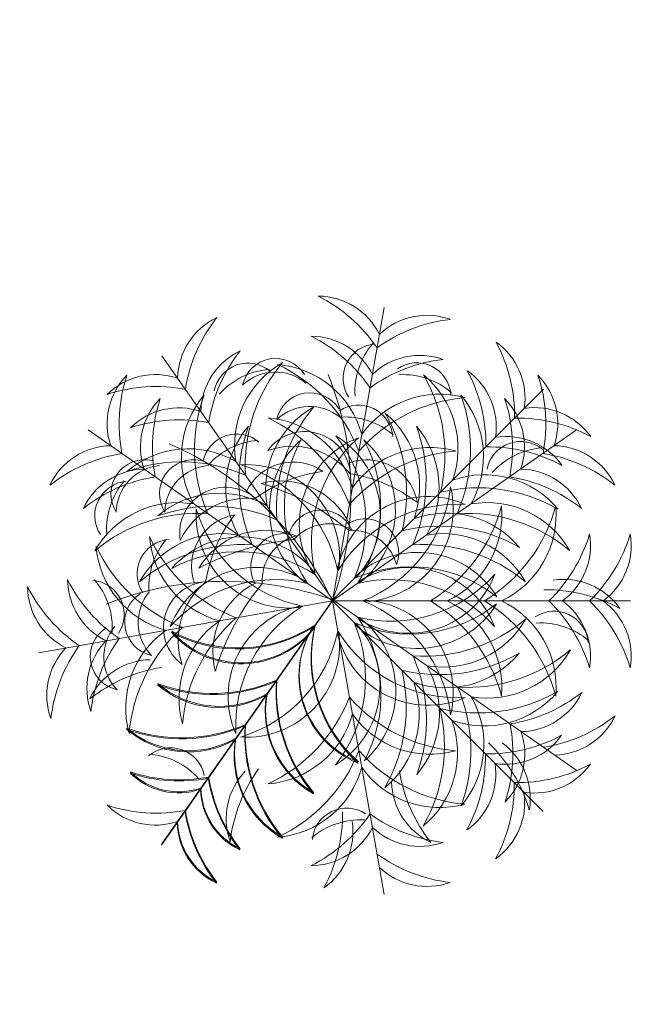
# Model space of a CAD drawing. Units: inches. Extents: x -48 to 50072, y 0 to 21068.
# Tile 14 of 75: x 236 to 263, y 305 to 347. Entities that reach past the tile are written whole.
import ezdxf

# ---------------------------------------------------------------- set-up
doc = ezdxf.new("R2010")
doc.units = ezdxf.units.IN
doc.header["$MEASUREMENT"] = 0
doc.layers.add('A-ANNO-DIMS', color=2, linetype='Continuous', lineweight=18)
doc.layers.add('L-PLNT', color=94, linetype='Continuous', lineweight=13)
doc.styles.get("Standard").update_dxf_attribs({"font": 'arial.ttf'})
doc.dimstyles.get("Standard").update_dxf_attribs({"dimtxt": 8, "dimasz": 0.18, "dimexe": 0.18, "dimexo": 0.0625, "dimgap": 0.09, "dimtad": 0, "dimtih": 1, "dimtoh": 1, "dimdec": 1, "dimzin": 0, "dimdsep": 46, "dimlunit": 4, "dimtxsty": 'Standard', "dimblk": 'ARCHTICK', "dimcen": 0.09, "dimadec": 0, "dimazin": 0, "dimtfac": 1, "dimtdec": 1, "dimtofl": 0, "dimtmove": 0, "dimatfit": 3, "dimldrblk": 'ARCHTICK', "dimfxl": 1, "dimtolj": 1, "dimtzin": 0, "dimarcsym": 0})

# ---------------------------------------------------------------- blocks, each defined once
blk = doc.blocks.new('A$C5D061C3B')
for p, q in [((3.377, 6.679), (3.377, 3.377)), ((1.483, 6.082), (3.377, 3.377)), ((5.259, 6.086), (3.365, 3.381)), ((1.03, 5.716), (3.365, 3.381)), ((5.712, 5.712), (3.377, 3.377)), ((0.125, 3.951), (3.377, 3.377)), ((6.629, 3.951), (3.377, 3.377)), ((0.66, 1.487), (3.365, 3.381)), ((1.483, 0.672), (3.377, 3.377)), ((6.07, 1.487), (3.365, 3.381)), ((3.951, 0.125), (3.377, 3.377)), ((6.082, 1.483), (3.377, 3.377))]:
    blk.add_line(p, q)
for centre, radius, start, end in [((2.763, 5.924), 0.762, 36.29, 99.6243), ((2.145, 5.032), 1.715, 44.0763, 73.3794), ((3.991, 5.924), 0.762, 80.3757, 143.71), ((4.61, 5.032), 1.715, 106.6206, 135.9237), ((3.901, 5.939), 0.762, 125.3757, 188.71), ((4.969, 5.745), 1.715, 151.6206, 180.9237), ((2.419, 5.816), 0.762, 115.3757, 178.71), ((3.438, 5.44), 1.715, 141.6206, 170.9237), ((3.305, 5.444), 1.715, 9.0763, 38.3794), ((4.323, 5.82), 0.762, 1.29, 64.6243), ((1.998, 5.617), 0.762, 125.3757, 188.71), ((3.066, 5.423), 1.715, 151.6206, 180.9237), ((2.763, 5.474), 0.762, 36.29, 99.6243), ((2.145, 4.581), 1.715, 44.0763, 73.3794), ((3.991, 5.474), 0.762, 80.3757, 143.71), ((4.61, 4.581), 1.715, 106.6206, 135.9237), ((4.744, 5.613), 0.762, 351.29, 54.6243), ((3.676, 5.419), 1.715, 359.0763, 28.3794), ((2.678, 5.447), 0.762, 115.3757, 178.71), ((3.696, 5.07), 1.715, 141.6206, 170.9237), ((3.871, 5.832), 0.38, 94.742, 213.7475), ((4.447, 5.681), 0.826, 139.618, 183.2106), ((4.064, 5.451), 0.762, 1.29, 64.6243), ((3.046, 5.075), 1.715, 9.0763, 38.3794), ((3.344, 5.089), 1.056, 119.6063, 189.7511), ((4.177, 4.869), 1.77, 139.9634, 183.6288), ((3.398, 5.094), 1.056, 350.2489, 60.3937), ((2.565, 4.873), 1.77, 356.3712, 40.0366), ((2.317, 5.298), 0.762, 125.3757, 188.71), ((3.385, 5.104), 1.715, 151.6206, 180.9237), ((3.357, 5.1), 1.715, 359.0763, 28.3794), ((4.425, 5.294), 0.762, 351.29, 54.6243), ((1.413, 5.111), 0.762, 71.29, 134.6243), ((3.035, 5.062), 1.056, 129.6063, 199.7511), ((3.894, 4.989), 1.77, 149.9634, 193.6288), ((2.422, 4.799), 1.056, 25.2489, 95.3937), ((1.866, 4.14), 1.77, 31.3712, 75.0366), ((4.332, 4.799), 1.056, 84.6063, 154.7511), ((4.888, 4.14), 1.77, 104.9634, 148.6288), ((2.848, 4.985), 1.77, 346.3712, 30.0366), ((3.707, 5.058), 1.056, 340.2489, 50.3937), ((1.419, 4.026), 1.715, 79.0763, 108.3794), ((1.991, 5.462), 0.38, 139.742, 258.7475), ((2.505, 5.763), 0.826, 184.618, 228.2106), ((5.564, 4.807), 0.762, 80.3757, 143.71), ((1.13, 4.748), 0.762, 81.29, 144.6243), ((1.671, 4.742), 0.762, 71.29, 134.6243), ((3.688, 4.597), 1.056, 119.6063, 189.7511), ((4.522, 4.377), 1.77, 139.9634, 183.6288), ((2.221, 4.381), 1.77, 356.3712, 40.0366), ((3.054, 4.602), 1.056, 350.2489, 60.3937), ((5.071, 4.746), 0.762, 45.3757, 108.71), ((6.182, 3.914), 1.715, 106.6206, 135.9237), ((5.613, 4.744), 0.762, 35.3757, 98.71), ((1.324, 3.68), 1.715, 89.0763, 118.3794), ((1.677, 3.657), 1.715, 79.0763, 108.3794), ((3.46, 4.637), 1.056, 129.6063, 199.7511), ((4.319, 4.565), 1.77, 149.9634, 193.6288), ((3.283, 4.633), 1.056, 340.2489, 50.3937), ((2.424, 4.56), 1.77, 346.3712, 30.0366), ((5.065, 3.661), 1.715, 71.6206, 100.9237), ((5.419, 3.676), 1.715, 61.6206, 90.9237), ((2.422, 4.198), 1.056, 25.2489, 95.3937), ((1.866, 3.54), 1.77, 31.3712, 75.0366), ((4.332, 4.198), 1.056, 84.6063, 154.7511), ((4.888, 3.54), 1.77, 104.9634, 148.6288), ((1.448, 4.43), 0.762, 81.29, 144.6243), ((3.868, 4.321), 1.029, 121.3654, 221.5741), ((4.556, 4.237), 1.557, 141.8122, 203.3335), ((4.035, 4.215), 1.029, 111.3654, 211.5741), ((2.707, 4.219), 1.029, 328.4259, 68.6346), ((2.044, 4.017), 1.557, 346.6665, 48.1878), ((4.698, 4.013), 1.557, 131.8122, 193.3335), ((2.187, 4.233), 1.557, 336.6665, 38.1878), ((2.875, 4.316), 1.029, 318.4259, 58.6346), ((5.294, 4.425), 0.762, 35.3757, 98.71), ((1.642, 3.362), 1.715, 89.0763, 118.3794), ((1.78, 3.994), 1.056, 60.2489, 130.3937), ((4.963, 3.998), 1.056, 49.6063, 119.7511), ((5.1, 3.357), 1.715, 61.6206, 90.9237), ((5.04, 3.14), 1.77, 69.9634, 113.6288), ((2.143, 4.564), 1.056, 164.6063, 234.7511), ((1.702, 3.136), 1.77, 66.3712, 110.0366), ((2.888, 4.998), 1.77, 184.9634, 228.6288), ((3.25, 4.435), 1.029, 156.3654, 256.5741), ((3.862, 4.761), 1.557, 176.8122, 238.3335), ((2.893, 4.761), 1.557, 301.6665, 3.1878), ((3.504, 4.435), 1.029, 283.4259, 23.6346), ((3.866, 4.998), 1.77, 311.3712, 355.0366), ((4.611, 4.564), 1.056, 305.2489, 15.3937), ((1.696, 4.159), 0.826, 139.618, 183.2106), ((1.685, 3.712), 1.056, 70.2489, 140.3937), ((2.734, 4.46), 1.056, 164.6063, 234.7511), ((3.48, 4.893), 1.77, 184.9634, 228.6288), ((2.358, 3.686), 1.029, 3.4259, 103.6346), ((4.397, 3.686), 1.029, 76.3654, 176.5741), ((3.275, 4.893), 1.77, 311.3712, 355.0366), ((4.02, 4.46), 1.056, 305.2489, 15.3937), ((5.058, 3.707), 1.056, 39.6063, 109.7511), ((0.975, 4.424), 0.762, 160.3757, 223.71), ((1.962, 4.878), 1.715, 186.6206, 215.9237), ((1.419, 4.346), 0.762, 160.3757, 223.71), ((2.405, 4.8), 1.715, 186.6206, 215.9237), ((1.12, 4.31), 0.38, 94.742, 213.7475), ((1.757, 2.853), 1.77, 76.3712, 120.0366), ((1.93, 3.14), 1.557, 21.6665, 83.1878), ((4.824, 3.14), 1.557, 96.8122, 158.3335), ((4.985, 2.848), 1.77, 59.9634, 103.6288), ((4.349, 4.8), 1.715, 324.0763, 353.3794), ((5.335, 4.346), 0.762, 316.29, 19.6243), ((4.793, 4.878), 1.715, 324.0763, 353.3794), ((5.779, 4.424), 0.762, 316.29, 19.6243), ((2.124, 3.502), 1.056, 60.2489, 130.3937), ((4.618, 3.506), 1.056, 49.6063, 119.7511), ((2.046, 2.644), 1.77, 66.3712, 110.0366), ((4.696, 2.648), 1.77, 69.9634, 113.6288), ((4.988, 5.812), 1.715, 279.0763, 308.3794), ((5.365, 4.794), 0.762, 271.29, 334.6243), ((2.109, 3.287), 1.056, 70.2489, 140.3937), ((2.387, 3.752), 0.574, 99.9865, 199.4034), ((3.599, 3.314), 1.651, 142.5759, 170.8942), ((4.633, 3.283), 1.056, 39.6063, 109.7511), ((2.182, 2.428), 1.77, 76.3712, 120.0366), ((4.56, 2.424), 1.77, 59.9634, 103.6288), ((1.588, 3.666), 0.38, 94.742, 213.7475), ((2.165, 3.515), 0.826, 139.618, 183.2106), ((2.365, 3.045), 1.029, 38.4259, 138.6346), ((2.84, 3.739), 0.372, 69.2257, 210.1279), ((3.109, 3.59), 0.515, 105.4398, 183.6694), ((4.377, 3.05), 1.029, 41.3654, 141.5741), ((0.762, 3.214), 0.762, 116.29, 179.6243), ((1.534, 2.451), 1.715, 124.0763, 153.3794), ((1.206, 3.136), 0.762, 116.29, 179.6243), ((1.062, 4.452), 0.826, 229.618, 273.2106), ((0.91, 3.875), 0.38, 184.742, 303.7475), ((2.426, 2.879), 1.029, 48.4259, 148.6346), ((2.328, 2.353), 1.557, 56.6665, 118.1878), ((4.414, 2.358), 1.557, 61.8122, 123.3335), ((4.316, 2.875), 1.029, 31.3654, 131.5741), ((5.549, 3.136), 0.762, 0.3757, 63.71), ((1.977, 2.373), 1.715, 124.0763, 153.3794), ((2.51, 2.191), 1.557, 66.6665, 128.1878), ((4.233, 2.187), 1.557, 51.8122, 113.3335), ((6.053, 3.533), 0.38, 146.2525, 265.258), ((4.777, 2.373), 1.715, 26.6206, 55.9237), ((6.629, 3.684), 0.826, 176.7894, 220.382), ((1.811, 2.684), 1.056, 105.2489, 175.3937), ((2.363, 2.022), 1.77, 111.3712, 155.0366), ((2.729, 4.702), 1.557, 221.8122, 283.3335), ((2.527, 4.039), 1.029, 201.3654, 301.5741), ((4.001, 4.702), 1.557, 256.6665, 318.1878), ((4.013, 4.698), 1.557, 256.6665, 318.1878), ((4.203, 4.039), 1.029, 238.4259, 338.6346), ((4.215, 4.035), 1.029, 238.4259, 338.6346), ((4.391, 2.022), 1.77, 24.9634, 68.6288), ((4.943, 2.684), 1.056, 4.6063, 74.7511), ((5.935, 2.842), 0.762, 35.3757, 98.71), ((2.185, 0.015), 3.567, 70.4772, 111.6585), ((2.403, 2.58), 1.056, 105.2489, 175.3937), ((2.955, 1.917), 1.77, 111.3712, 155.0366), ((2.007, 3.071), 0.506, 93.8744, 233.9763), ((2.489, 2.932), 0.825, 128.7536, 199.097), ((2.903, 2.8), 0.855, 116.4477, 194.3672), ((4.744, 1.779), 2.789, 140.4007, 163.139), ((2.741, 3.253), 0.372, 114.2257, 255.1279), ((3.037, 3.338), 0.515, 150.4398, 228.6694), ((3.799, 1.917), 1.77, 24.9634, 68.6288), ((4.352, 2.58), 1.056, 4.6063, 74.7511), ((1.447, 3.129), 0.376, 122.0577, 257.8533), ((1.751, 3.126), 0.529, 140.1845, 223.654), ((2.896, 2.427), 1.029, 83.4259, 183.6346), ((3.359, 1.911), 1.557, 101.6665, 163.1878), ((3.395, 1.911), 1.557, 16.8122, 78.3335), ((3.858, 2.427), 1.029, 356.3654, 96.5741), ((5.741, 1.774), 1.715, 61.6206, 90.9237), ((4.912, 0.157), 3.567, 115.4772, 156.6585), ((6.727, 2.189), 3.567, 160.4772, 201.6585), ((2.145, 3.693), 1.056, 209.6063, 279.7511), ((2.365, 4.526), 1.77, 229.9634, 273.6288), ((2.412, 2.943), 0.574, 144.9865, 244.4034), ((3.578, 3.49), 1.651, 187.5759, 215.8942), ((3.697, 2.369), 1.029, 128.4259, 228.6346), ((4.389, 2.332), 1.557, 146.6665, 208.1878), ((2.341, 2.332), 1.557, 331.8122, 33.3335), ((2.353, 2.328), 1.557, 331.8122, 33.3335), ((3.033, 2.369), 1.029, 311.3654, 51.5741), ((3.045, 2.365), 1.029, 311.3654, 51.5741), ((4.365, 4.526), 1.77, 266.3712, 310.0366), ((4.377, 4.522), 1.77, 266.3712, 310.0366), ((4.585, 3.693), 1.056, 260.2489, 330.3937), ((4.597, 3.688), 1.056, 260.2489, 330.3937), ((1.067, 2.749), 0.376, 122.0577, 257.8533), ((1.37, 2.745), 0.529, 140.1845, 223.654), ((2.328, 4.401), 1.557, 241.8122, 303.3335), ((2.365, 3.709), 1.029, 221.3654, 321.5741), ((4.035, 2.539), 1.029, 148.4259, 248.6346), ((4.698, 2.741), 1.557, 166.6665, 228.1878), ((1.911, 3.359), 1.557, 286.8122, 348.3335), ((2.427, 2.896), 1.029, 266.3654, 6.5741), ((3.003, 2.844), 0.372, 159.2257, 300.1279), ((3.152, 3.113), 0.515, 195.4398, 273.6694), ((5.474, 3.214), 2.789, 185.4007, 208.139), ((4.435, 3.25), 1.029, 193.4259, 293.6346), ((4.761, 3.862), 1.557, 211.6665, 273.1878), ((3.45, 2.634), 0.855, 161.4477, 239.3672), ((1.873, 4.181), 1.77, 229.9634, 273.6288), ((1.653, 3.348), 1.056, 209.6063, 279.7511), ((4.099, 2.051), 1.77, 156.3712, 200.0366), ((2.632, 2.051), 1.77, 339.9634, 23.6288), ((2.644, 2.046), 1.77, 339.9634, 23.6288), ((4.857, 4.181), 1.77, 266.3712, 310.0366), ((4.869, 4.177), 1.77, 266.3712, 310.0366), ((5.077, 3.348), 1.056, 260.2489, 330.3937), ((5.089, 3.344), 1.056, 260.2489, 330.3937), ((1.122, 2.441), 0.38, 139.742, 258.7475), ((1.636, 2.741), 0.826, 184.618, 228.2106), ((3.24, 2.128), 1.056, 150.2489, 220.3937), ((3.49, 2.128), 1.056, 319.6063, 29.7511), ((3.502, 2.124), 1.056, 319.6063, 29.7511), ((1.908, 2.317), 0.38, 139.742, 258.7475), ((2.422, 2.617), 0.826, 184.618, 228.2106), ((2.624, 2.192), 0.506, 138.8744, 278.9763), ((3.064, 2.435), 0.825, 173.7536, 244.097), ((3.942, 2.908), 0.855, 206.4477, 284.3672), ((4.963, 4.749), 2.789, 230.4007, 253.139), ((6.244, 3.948), 1.715, 234.0763, 263.3794), ((2.046, 4.111), 1.77, 249.9634, 293.6288), ((2.124, 3.252), 1.056, 229.6063, 299.7511), ((3.607, 1.706), 1.77, 156.3712, 200.0366), ((4.522, 2.378), 1.77, 176.3712, 220.0366), ((3.124, 1.706), 1.77, 339.9634, 23.6288), ((3.136, 1.702), 1.77, 339.9634, 23.6288), ((5.79, 2.962), 0.762, 226.29, 289.6243), ((1.672, 3.7), 1.715, 231.6206, 260.9237), ((1.295, 2.682), 0.762, 205.3757, 268.71), ((2.748, 1.784), 1.056, 150.2489, 220.3937), ((3.428, 3.603), 1.651, 232.5759, 260.8942), ((2.99, 2.391), 0.574, 189.9865, 289.4034), ((3.688, 2.157), 1.056, 170.2489, 240.3937), ((1.917, 2.955), 1.77, 294.9634, 338.6288), ((4.893, 3.48), 1.77, 221.3712, 265.0366), ((3.982, 1.784), 1.056, 319.6063, 29.7511), ((3.994, 1.78), 1.056, 319.6063, 29.7511), ((5.058, 3.7), 1.715, 279.0763, 308.3794), ((5.07, 3.696), 1.715, 279.0763, 308.3794), ((5.435, 2.682), 0.762, 271.29, 334.6243), ((5.447, 2.678), 0.762, 271.29, 334.6243), ((0.926, 2.424), 0.762, 205.3757, 268.71), ((1.303, 3.442), 1.715, 231.6206, 260.9237), ((2.58, 2.403), 1.056, 274.6063, 344.7511), ((4.46, 2.734), 1.056, 215.2489, 285.3937), ((5.427, 3.442), 1.715, 279.0763, 308.3794), ((5.44, 3.438), 1.715, 279.0763, 308.3794), ((5.804, 2.424), 0.762, 271.29, 334.6243), ((5.816, 2.419), 0.762, 271.29, 334.6243), ((1.702, 3.619), 1.77, 249.9634, 293.6288), ((3.086, 1.681), 1.715, 169.0763, 198.3794), ((2.405, 2.049), 0.529, 185.1845, 268.654), ((4.177, 1.886), 1.77, 176.3712, 220.0366), ((3.81, 2.493), 0.825, 218.7536, 289.097), ((3.671, 2.011), 0.506, 183.8744, 323.9763), ((3.645, 1.681), 1.715, 341.6206, 10.9237), ((3.657, 1.677), 1.715, 341.6206, 10.9237), ((1.78, 2.76), 1.056, 229.6063, 299.7511), ((2, 1.676), 0.762, 161.29, 224.6243), ((2.188, 1.837), 0.376, 167.0577, 302.8533), ((5.385, 1.584), 0.38, 101.2525, 220.258), ((5.899, 1.283), 0.826, 131.7894, 175.382), ((4.73, 1.676), 0.762, 315.3757, 18.71), ((4.742, 1.671), 0.762, 315.3757, 18.71), ((2.717, 1.423), 1.715, 169.0763, 198.3794), ((3.344, 1.665), 1.056, 170.2489, 240.3937), ((4.014, 1.423), 1.715, 341.6206, 10.9237), ((1.631, 1.417), 0.762, 161.29, 224.6243), ((2.022, 2.363), 1.77, 294.9634, 338.6288), ((4.998, 2.888), 1.77, 221.3712, 265.0366), ((5.099, 1.417), 0.762, 315.3757, 18.71), ((3.227, 2.169), 0.826, 229.618, 273.2106), ((3.076, 1.593), 0.38, 184.742, 303.7475), ((2.684, 1.811), 1.056, 274.6063, 344.7511), ((4.564, 2.143), 1.056, 215.2489, 285.3937), ((1.671, 2.012), 0.762, 225.3757, 288.71), ((1.677, 3.098), 1.715, 251.6206, 280.9237), ((2.405, 1.511), 0.529, 185.1845, 268.654), ((5.808, 1.754), 1.715, 189.0763, 218.3794), ((2.188, 1.299), 0.376, 167.0577, 302.8533), ((3.696, 1.684), 1.715, 189.0763, 218.3794), ((3.616, 1.755), 0.529, 230.1845, 313.654), ((3.613, 1.452), 0.376, 212.0577, 347.8533), ((4.79, 1.377), 0.762, 181.29, 244.6243), ((2.678, 1.307), 0.762, 181.29, 244.6243), ((1.419, 2.729), 1.715, 251.6206, 280.9237), ((1.413, 1.643), 0.762, 225.3757, 288.71), ((2.432, 1.124), 0.38, 184.742, 303.7475), ((3.438, 1.315), 1.715, 189.0763, 218.3794), ((2.583, 1.701), 0.826, 229.618, 273.2106), ((2.373, 1.977), 1.715, 296.6206, 325.9237), ((3.528, 0.69), 0.38, 56.2525, 175.258), ((3.997, 1.374), 0.529, 230.1845, 313.654), ((3.994, 1.071), 0.376, 212.0577, 347.8533), ((4.8, 2.405), 1.715, 234.0763, 263.3794), ((2.419, 0.938), 0.762, 181.29, 244.6243), ((3.68, 0.113), 0.826, 86.7894, 130.382), ((3.136, 1.206), 0.762, 270.3757, 333.71), ((4.346, 1.419), 0.762, 226.29, 289.6243), ((2.451, 1.534), 1.715, 296.6206, 325.9237), ((4.878, 1.962), 1.715, 234.0763, 263.3794), ((3.214, 0.762), 0.762, 270.3757, 333.71), ((4.424, 0.975), 0.762, 226.29, 289.6243)]:
    blk.add_arc(centre, radius, start, end)
blk = doc.blocks.new('_ArchTick')
at = {"color": 0, "linetype": 'ByBlock', "const_width": 0.15}
blk.add_lwpolyline([(-0.5, -0.5), (0.5, 0.5)], dxfattribs=at)
blk = doc.blocks.new('*D117')
at = {"layer": 'A-ANNO-DIMS', "color": 0, "lineweight": -2, "transparency": 16777216}
for p, q in [((216.017, 488.712), (216.017, 165.945)), ((297.017, 488.712), (297.017, 165.945)), ((216.017, 166.125), (251.464, 166.125)), ((297.017, 166.125), (261.57, 166.125))]:
    blk.add_line(p, q, dxfattribs=at)
at = {"layer": 'Defpoints', "color": 0, "transparency": 16777216}
for p in [(216.017, 488.775), (297.017, 488.775), (297.017, 166.125)]:
    blk.add_point(p, dxfattribs=at)
at = {"layer": 'A-ANNO-DIMS', "color": 0, "lineweight": -2, "transparency": 16777216, "xscale": 0.18, "yscale": 0.18, "zscale": 0.18, "rotation": 180}
blk.add_blockref('_ArchTick', (216.017, 166.125), dxfattribs=at)
at = {"layer": 'A-ANNO-DIMS', "color": 0, "lineweight": -2, "transparency": 16777216, "xscale": 0.18, "yscale": 0.18, "zscale": 0.18}
blk.add_blockref('_ArchTick', (297.017, 166.125), dxfattribs=at)
at = {"layer": 'A-ANNO-DIMS', "color": 0, "transparency": 16777216, "insert": (256.517, 166.125), "char_height": 8, "attachment_point": 5}
blk.add_mtext('\\A1;81', dxfattribs=at)

msp = doc.modelspace()

# ---------------------------------------------------------------- block references
at = {"layer": 'L-PLNT', "xscale": 3.862191520948588, "yscale": 3.862191520948588, "zscale": 3.862191520948588, "rotation": 270}
msp.add_blockref('A$C5D061C3B', (236.199, 335.479), dxfattribs=at)

# ---------------------------------------------------------------- dimensions: what is measured, and where the dimension line sits
at = {"layer": 'A-ANNO-DIMS'}
dim = msp.add_linear_dim(base=(297.017, 166.125), p1=(216.017, 488.775), p2=(297.017, 488.775), dimstyle='Standard', override={"dimdec": 0, "dimlfac": 1, "dimrnd": 0, "dimzin": 0, "dimdsep": 46, "dimlunit": 2}, dxfattribs=at)
dim.commit()
dim.dimension.update_dxf_attribs({"geometry": '*D117', "text_midpoint": (256.517, 166.125)})

doc.saveas('drawing.dxf')
